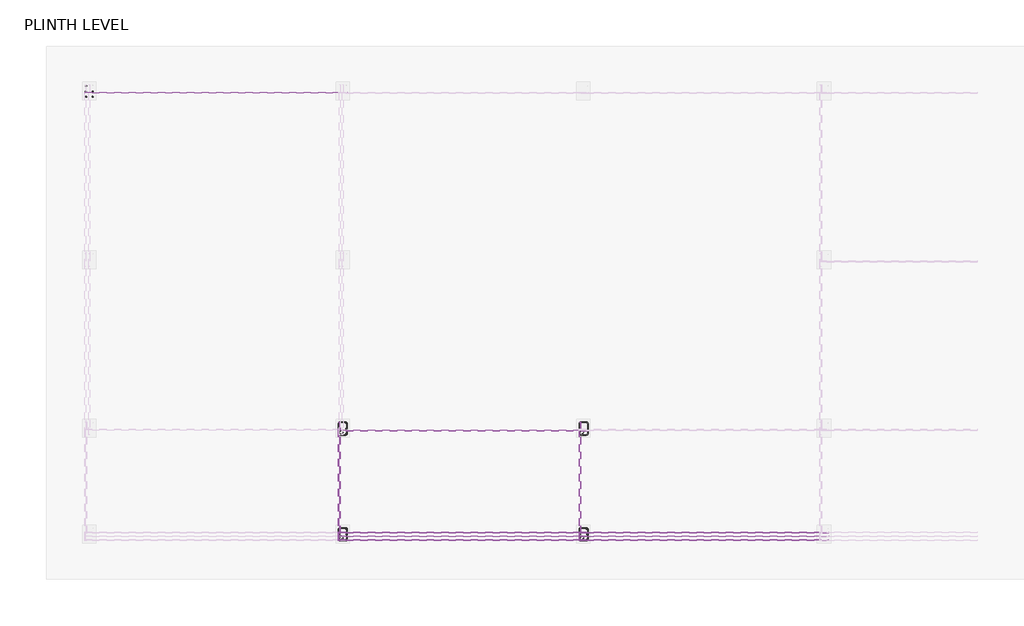
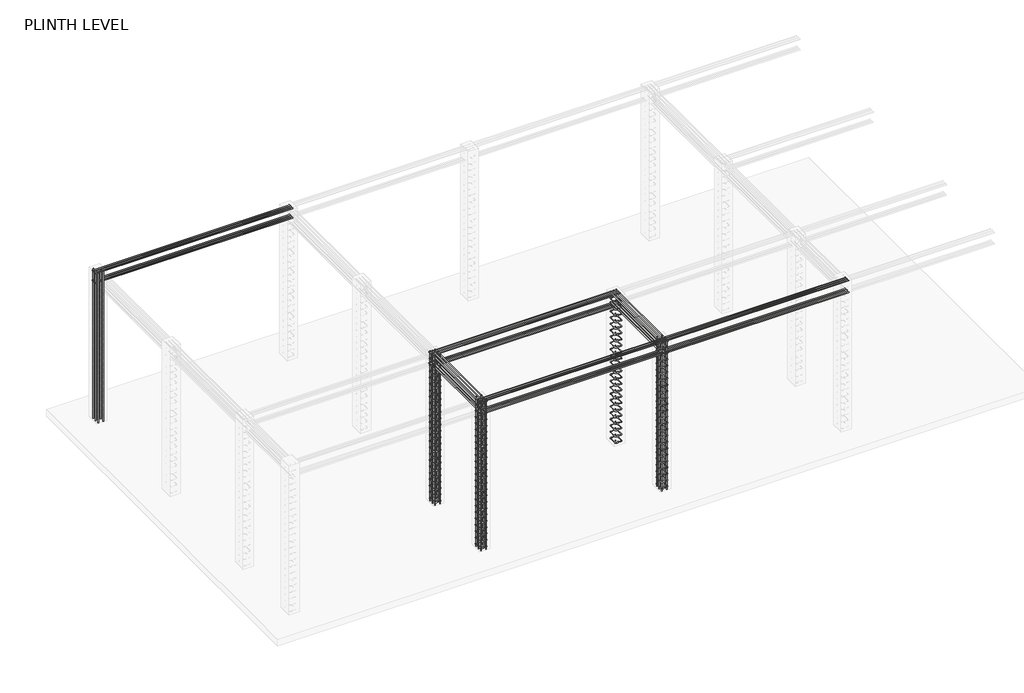
# One storey, part 3 of 6: 47 reinforcing bars.
"""IFC4 building model written with IfcOpenShell, lengths in millimetres."""

from ifc_helpers import new_model, si_unit, point, frame, origin, place, context, project, spatial, polyline, circle_curve, trimmed, segment, composite_curve, source, transform, mapped, element, save
from ifc_brep_helpers import swept_disk

model = new_model("IFC4")

# Units and contexts
model_context = context("Model", 3, world=origin())
ifc_project = project(units=[si_unit("LENGTHUNIT", "METRE", prefix="MILLI")], contexts=[model_context])

# Site, building, storey
site = spatial("IfcSite", under=ifc_project)
building = spatial("IfcBuilding", under=site)
storey = spatial("IfcBuildingStorey", under=building, Name="PLINTH LEVEL", Elevation=0.0)

# Reinforcing bars
placement = place(None, origin())
reinforcing_bar_shape = source(origin(), model_context, "Body", "SolidModel", [
    swept_disk(composite_curve([segment(polyline([(1580.248777, -15125.7150493, 44.0), (1546.3076515, -15159.6561748, 44.0)]), True, "CONTINUOUS"), segment(trimmed(circle_curve(frame((1563.2782143, -15176.6267376, 44.0), z_axis=(0.0, 0.0, 1.0), x_axis=(-16.970562799999925, 16.970562799999243, 0.0)), 24.0), [point((1546.3076515, -15159.6561748, 44.0))], [point((1563.2782143, -15200.6267376, 44.0))], True, "CARTESIAN"), True, "CONTINUOUS"), segment(polyline([(1563.2782143, -15200.6267376, 44.0), (1657.2782143, -15200.6267376, 44.0)]), True, "CONTINUOUS"), segment(trimmed(circle_curve(frame((1657.2782143, -15176.6267376, 44.0), z_axis=(0.0, 0.0, 1.0), x_axis=(0.0, -24.0, 0.0)), 24.0), [point((1657.2782143, -15200.6267376, 44.0))], [point((1681.2782143, -15176.6267376, 44.0))], True, "CARTESIAN"), True, "CONTINUOUS"), segment(polyline([(1681.2782143, -15176.6267376, 44.0), (1681.2782143, -15012.6267376, 44.0)]), True, "CONTINUOUS"), segment(trimmed(circle_curve(frame((1657.3162115, -15012.6267376, 42.650028), z_axis=(-0.05624883273897079, 0.0, 0.9984167811167355), x_axis=(23.962002799999937, 0.0, 1.349972000000001)), 24.0), [point((1681.2782143, -15012.6267376, 44.0))], [point((1657.3162115, -14988.6267376, 42.650028))], True, "CARTESIAN"), True, "CONTINUOUS"), segment(polyline([(1657.3162115, -14988.6267376, 42.650028), (1563.240217, -14988.6267376, 37.349972)]), True, "CONTINUOUS"), segment(trimmed(circle_curve(frame((1563.240217, -15012.6267376, 37.349972), z_axis=(-0.05624883273897079, 0.0, 0.9984167811167355), x_axis=(0.0, 24.0, 0.0)), 24.0), [point((1563.240217, -14988.6267376, 37.349972))], [point((1539.2782143, -15012.6267376, 36.0))], True, "CARTESIAN"), True, "CONTINUOUS"), segment(polyline([(1539.2782143, -15012.6267376, 36.0), (1539.2782143, -15176.6267376, 36.0)]), True, "CONTINUOUS"), segment(trimmed(circle_curve(frame((1563.2782143, -15176.6267376, 36.0), z_axis=(0.0, 0.0, 1.0), x_axis=(-24.0, 0.0, 0.0)), 24.0), [point((1539.2782143, -15176.6267376, 36.0))], [point((1580.248777, -15193.5973003, 36.0))], True, "CARTESIAN"), True, "CONTINUOUS"), segment(polyline([(1580.248777, -15193.5973003, 36.0), (1614.1899025, -15159.6561748, 36.0)]), True, "CONTINUOUS")], self_intersect=False), 4.0),
])
element("IfcReinforcingBar", 1, at=placement, inside=storey, context=model_context, shape_type="MappedRepresentation", body=[
    mapped(reinforcing_bar_shape, transform((0.0, 0.0, 0.0), x_axis=(1.0, 0.0, 0.0), y_axis=(0.0, 1.0, 0.0), z_axis=(0.0, 0.0, 1.0))),
    mapped(reinforcing_bar_shape, transform((0.0, 0.0, 149.0483786), x_axis=(1.0, 0.0, 0.0), y_axis=(0.0, 1.0, 0.0), z_axis=(0.0, 0.0, 1.0))),
    mapped(reinforcing_bar_shape, transform((0.0, 0.0, 298.0967572), x_axis=(1.0, 0.0, 0.0), y_axis=(0.0, 1.0, 0.0), z_axis=(0.0, 0.0, 1.0))),
    mapped(reinforcing_bar_shape, transform((0.0, 0.0, 447.1451358), x_axis=(1.0, 0.0, 0.0), y_axis=(0.0, 1.0, 0.0), z_axis=(0.0, 0.0, 1.0))),
    mapped(reinforcing_bar_shape, transform((0.0, 0.0, 596.1935144), x_axis=(1.0, 0.0, 0.0), y_axis=(0.0, 1.0, 0.0), z_axis=(0.0, 0.0, 1.0))),
    mapped(reinforcing_bar_shape, transform((0.0, 0.0, 745.241893), x_axis=(1.0, 0.0, 0.0), y_axis=(0.0, 1.0, 0.0), z_axis=(0.0, 0.0, 1.0))),
    mapped(reinforcing_bar_shape, transform((0.0, 0.0, 894.2902717), x_axis=(1.0, 0.0, 0.0), y_axis=(0.0, 1.0, 0.0), z_axis=(0.0, 0.0, 1.0))),
    mapped(reinforcing_bar_shape, transform((0.0, 0.0, 1043.3386503), x_axis=(1.0, 0.0, 0.0), y_axis=(0.0, 1.0, 0.0), z_axis=(0.0, 0.0, 1.0))),
    mapped(reinforcing_bar_shape, transform((0.0, 0.0, 1192.3870289), x_axis=(1.0, 0.0, 0.0), y_axis=(0.0, 1.0, 0.0), z_axis=(0.0, 0.0, 1.0))),
    mapped(reinforcing_bar_shape, transform((0.0, 0.0, 1341.4354075), x_axis=(1.0, 0.0, 0.0), y_axis=(0.0, 1.0, 0.0), z_axis=(0.0, 0.0, 1.0))),
    mapped(reinforcing_bar_shape, transform((0.0, 0.0, 1490.4837861), x_axis=(1.0, 0.0, 0.0), y_axis=(0.0, 1.0, 0.0), z_axis=(0.0, 0.0, 1.0))),
    mapped(reinforcing_bar_shape, transform((0.0, 0.0, 1639.5321647), x_axis=(1.0, 0.0, 0.0), y_axis=(0.0, 1.0, 0.0), z_axis=(0.0, 0.0, 1.0))),
    mapped(reinforcing_bar_shape, transform((0.0, 0.0, 1788.5805433), x_axis=(1.0, 0.0, 0.0), y_axis=(0.0, 1.0, 0.0), z_axis=(0.0, 0.0, 1.0))),
    mapped(reinforcing_bar_shape, transform((0.0, 0.0, 1937.6289219), x_axis=(1.0, 0.0, 0.0), y_axis=(0.0, 1.0, 0.0), z_axis=(0.0, 0.0, 1.0))),
    mapped(reinforcing_bar_shape, transform((0.0, 0.0, 2086.6773005), x_axis=(1.0, 0.0, 0.0), y_axis=(0.0, 1.0, 0.0), z_axis=(0.0, 0.0, 1.0))),
    mapped(reinforcing_bar_shape, transform((0.0, 0.0, 2235.7256791), x_axis=(1.0, 0.0, 0.0), y_axis=(0.0, 1.0, 0.0), z_axis=(0.0, 0.0, 1.0))),
    mapped(reinforcing_bar_shape, transform((0.0, 0.0, 2384.7740578), x_axis=(1.0, 0.0, 0.0), y_axis=(0.0, 1.0, 0.0), z_axis=(0.0, 0.0, 1.0))),
    mapped(reinforcing_bar_shape, transform((0.0, 0.0, 2533.8224364), x_axis=(1.0, 0.0, 0.0), y_axis=(0.0, 1.0, 0.0), z_axis=(0.0, 0.0, 1.0))),
    mapped(reinforcing_bar_shape, transform((0.0, 0.0, 2682.870815), x_axis=(1.0, 0.0, 0.0), y_axis=(0.0, 1.0, 0.0), z_axis=(0.0, 0.0, 1.0))),
    mapped(reinforcing_bar_shape, transform((0.0, 0.0, 2831.9191936), x_axis=(1.0, 0.0, 0.0), y_axis=(0.0, 1.0, 0.0), z_axis=(0.0, 0.0, 1.0))),
    mapped(reinforcing_bar_shape, transform((0.0, 0.0, 2980.9675722), x_axis=(1.0, 0.0, 0.0), y_axis=(0.0, 1.0, 0.0), z_axis=(0.0, 0.0, 1.0))),
    mapped(reinforcing_bar_shape, transform((0.0, 0.0, 3130.0159508), x_axis=(1.0, 0.0, 0.0), y_axis=(0.0, 1.0, 0.0), z_axis=(0.0, 0.0, 1.0))),
    mapped(reinforcing_bar_shape, transform((0.0, 0.0, 3279.0643294), x_axis=(1.0, 0.0, 0.0), y_axis=(0.0, 1.0, 0.0), z_axis=(0.0, 0.0, 1.0))),
])
element("IfcReinforcingBar", 2, at=placement, inside=storey, context=model_context, shape_type="SolidModel", body=[
    swept_disk(composite_curve([segment(polyline([(1665.7634957, -15004.1414562, -20.0), (1665.7634957, -15004.1414562, 3485.2)]), True, "CONTINUOUS")], self_intersect=False), 8.0),
])
element("IfcReinforcingBar", 3, at=placement, inside=storey, context=model_context, shape_type="SolidModel", body=[
    swept_disk(composite_curve([segment(polyline([(1665.7634957, -15185.112019, -20.0), (1665.7634957, -15185.112019, 3485.2)]), True, "CONTINUOUS")], self_intersect=False), 8.0),
])
element("IfcReinforcingBar", 4, at=placement, inside=storey, context=model_context, shape_type="SolidModel", body=[
    swept_disk(composite_curve([segment(polyline([(1669.2782143, -15094.6267376, -20.0), (1669.2782143, -15094.6267376, 3485.2)]), True, "CONTINUOUS")], self_intersect=False), 8.0),
])
element("IfcReinforcingBar", 5, at=placement, inside=storey, context=model_context, shape_type="SolidModel", body=[
    swept_disk(composite_curve([segment(polyline([(1554.7929329, -15004.1414562, -20.0), (1554.7929329, -15004.1414562, 3485.2)]), True, "CONTINUOUS")], self_intersect=False), 8.0),
])
element("IfcReinforcingBar", 6, at=placement, inside=storey, context=model_context, shape_type="SolidModel", body=[
    swept_disk(composite_curve([segment(polyline([(1554.7929329, -15185.112019, -20.0), (1554.7929329, -15185.112019, 3485.2)]), True, "CONTINUOUS")], self_intersect=False), 8.0),
])
element("IfcReinforcingBar", 7, at=placement, inside=storey, context=model_context, shape_type="SolidModel", body=[
    swept_disk(composite_curve([segment(polyline([(1551.2782143, -15094.6267376, -20.0), (1551.2782143, -15094.6267376, 3485.2)]), True, "CONTINUOUS")], self_intersect=False), 8.0),
])
reinforcing_bar_2_shape = source(origin(), model_context, "Body", "SolidModel", [
    swept_disk(composite_curve([segment(polyline([(5595.248777, -15125.7150493, 44.0), (5561.3076515, -15159.6561748, 44.0)]), True, "CONTINUOUS"), segment(trimmed(circle_curve(frame((5578.2782143, -15176.6267376, 44.0), z_axis=(0.0, 0.0, 1.0), x_axis=(-16.970562800000152, 16.970562799999243, 0.0)), 24.0), [point((5561.3076515, -15159.6561748, 44.0))], [point((5578.2782143, -15200.6267376, 44.0))], True, "CARTESIAN"), True, "CONTINUOUS"), segment(polyline([(5578.2782143, -15200.6267376, 44.0), (5672.2782143, -15200.6267376, 44.0)]), True, "CONTINUOUS"), segment(trimmed(circle_curve(frame((5672.2782143, -15176.6267376, 44.0), z_axis=(0.0, 0.0, 1.0), x_axis=(0.0, -24.0, 0.0)), 24.0), [point((5672.2782143, -15200.6267376, 44.0))], [point((5696.2782143, -15176.6267376, 44.0))], True, "CARTESIAN"), True, "CONTINUOUS"), segment(polyline([(5696.2782143, -15176.6267376, 44.0), (5696.2782143, -15012.6267376, 44.0)]), True, "CONTINUOUS"), segment(trimmed(circle_curve(frame((5672.3162115, -15012.6267376, 42.650028), z_axis=(-0.05624883273897079, 0.0, 0.9984167811167355), x_axis=(23.962002800000846, 0.0, 1.349972000000001)), 24.0), [point((5696.2782143, -15012.6267376, 44.0))], [point((5672.3162115, -14988.6267376, 42.650028))], True, "CARTESIAN"), True, "CONTINUOUS"), segment(polyline([(5672.3162115, -14988.6267376, 42.650028), (5578.240217, -14988.6267376, 37.349972)]), True, "CONTINUOUS"), segment(trimmed(circle_curve(frame((5578.240217, -15012.6267376, 37.349972), z_axis=(-0.05624883273897079, 0.0, 0.9984167811167355), x_axis=(0.0, 24.0, 0.0)), 24.0), [point((5578.240217, -14988.6267376, 37.349972))], [point((5554.2782143, -15012.6267376, 36.0))], True, "CARTESIAN"), True, "CONTINUOUS"), segment(polyline([(5554.2782143, -15012.6267376, 36.0), (5554.2782143, -15176.6267376, 36.0)]), True, "CONTINUOUS"), segment(trimmed(circle_curve(frame((5578.2782143, -15176.6267376, 36.0), z_axis=(0.0, 0.0, 1.0), x_axis=(-24.0, 0.0, 0.0)), 24.0), [point((5554.2782143, -15176.6267376, 36.0))], [point((5595.248777, -15193.5973003, 36.0))], True, "CARTESIAN"), True, "CONTINUOUS"), segment(polyline([(5595.248777, -15193.5973003, 36.0), (5629.1899025, -15159.6561748, 36.0)]), True, "CONTINUOUS")], self_intersect=False), 4.0),
])
element("IfcReinforcingBar", 8, at=placement, inside=storey, context=model_context, shape_type="MappedRepresentation", body=[
    mapped(reinforcing_bar_2_shape, transform((0.0, 0.0, 0.0), x_axis=(1.0, 0.0, 0.0), y_axis=(0.0, 1.0, 0.0), z_axis=(0.0, 0.0, 1.0))),
    mapped(reinforcing_bar_2_shape, transform((0.0, 0.0, 149.0483786), x_axis=(1.0, 0.0, 0.0), y_axis=(0.0, 1.0, 0.0), z_axis=(0.0, 0.0, 1.0))),
    mapped(reinforcing_bar_2_shape, transform((0.0, 0.0, 298.0967572), x_axis=(1.0, 0.0, 0.0), y_axis=(0.0, 1.0, 0.0), z_axis=(0.0, 0.0, 1.0))),
    mapped(reinforcing_bar_2_shape, transform((0.0, 0.0, 447.1451358), x_axis=(1.0, 0.0, 0.0), y_axis=(0.0, 1.0, 0.0), z_axis=(0.0, 0.0, 1.0))),
    mapped(reinforcing_bar_2_shape, transform((0.0, 0.0, 596.1935144), x_axis=(1.0, 0.0, 0.0), y_axis=(0.0, 1.0, 0.0), z_axis=(0.0, 0.0, 1.0))),
    mapped(reinforcing_bar_2_shape, transform((0.0, 0.0, 745.241893), x_axis=(1.0, 0.0, 0.0), y_axis=(0.0, 1.0, 0.0), z_axis=(0.0, 0.0, 1.0))),
    mapped(reinforcing_bar_2_shape, transform((0.0, 0.0, 894.2902717), x_axis=(1.0, 0.0, 0.0), y_axis=(0.0, 1.0, 0.0), z_axis=(0.0, 0.0, 1.0))),
    mapped(reinforcing_bar_2_shape, transform((0.0, 0.0, 1043.3386503), x_axis=(1.0, 0.0, 0.0), y_axis=(0.0, 1.0, 0.0), z_axis=(0.0, 0.0, 1.0))),
    mapped(reinforcing_bar_2_shape, transform((0.0, 0.0, 1192.3870289), x_axis=(1.0, 0.0, 0.0), y_axis=(0.0, 1.0, 0.0), z_axis=(0.0, 0.0, 1.0))),
    mapped(reinforcing_bar_2_shape, transform((0.0, 0.0, 1341.4354075), x_axis=(1.0, 0.0, 0.0), y_axis=(0.0, 1.0, 0.0), z_axis=(0.0, 0.0, 1.0))),
    mapped(reinforcing_bar_2_shape, transform((0.0, 0.0, 1490.4837861), x_axis=(1.0, 0.0, 0.0), y_axis=(0.0, 1.0, 0.0), z_axis=(0.0, 0.0, 1.0))),
    mapped(reinforcing_bar_2_shape, transform((0.0, 0.0, 1639.5321647), x_axis=(1.0, 0.0, 0.0), y_axis=(0.0, 1.0, 0.0), z_axis=(0.0, 0.0, 1.0))),
    mapped(reinforcing_bar_2_shape, transform((0.0, 0.0, 1788.5805433), x_axis=(1.0, 0.0, 0.0), y_axis=(0.0, 1.0, 0.0), z_axis=(0.0, 0.0, 1.0))),
    mapped(reinforcing_bar_2_shape, transform((0.0, 0.0, 1937.6289219), x_axis=(1.0, 0.0, 0.0), y_axis=(0.0, 1.0, 0.0), z_axis=(0.0, 0.0, 1.0))),
    mapped(reinforcing_bar_2_shape, transform((0.0, 0.0, 2086.6773005), x_axis=(1.0, 0.0, 0.0), y_axis=(0.0, 1.0, 0.0), z_axis=(0.0, 0.0, 1.0))),
    mapped(reinforcing_bar_2_shape, transform((0.0, 0.0, 2235.7256791), x_axis=(1.0, 0.0, 0.0), y_axis=(0.0, 1.0, 0.0), z_axis=(0.0, 0.0, 1.0))),
    mapped(reinforcing_bar_2_shape, transform((0.0, 0.0, 2384.7740578), x_axis=(1.0, 0.0, 0.0), y_axis=(0.0, 1.0, 0.0), z_axis=(0.0, 0.0, 1.0))),
    mapped(reinforcing_bar_2_shape, transform((0.0, 0.0, 2533.8224364), x_axis=(1.0, 0.0, 0.0), y_axis=(0.0, 1.0, 0.0), z_axis=(0.0, 0.0, 1.0))),
    mapped(reinforcing_bar_2_shape, transform((0.0, 0.0, 2682.870815), x_axis=(1.0, 0.0, 0.0), y_axis=(0.0, 1.0, 0.0), z_axis=(0.0, 0.0, 1.0))),
    mapped(reinforcing_bar_2_shape, transform((0.0, 0.0, 2831.9191936), x_axis=(1.0, 0.0, 0.0), y_axis=(0.0, 1.0, 0.0), z_axis=(0.0, 0.0, 1.0))),
    mapped(reinforcing_bar_2_shape, transform((0.0, 0.0, 2980.9675722), x_axis=(1.0, 0.0, 0.0), y_axis=(0.0, 1.0, 0.0), z_axis=(0.0, 0.0, 1.0))),
    mapped(reinforcing_bar_2_shape, transform((0.0, 0.0, 3130.0159508), x_axis=(1.0, 0.0, 0.0), y_axis=(0.0, 1.0, 0.0), z_axis=(0.0, 0.0, 1.0))),
    mapped(reinforcing_bar_2_shape, transform((0.0, 0.0, 3279.0643294), x_axis=(1.0, 0.0, 0.0), y_axis=(0.0, 1.0, 0.0), z_axis=(0.0, 0.0, 1.0))),
])
element("IfcReinforcingBar", 9, at=placement, inside=storey, context=model_context, shape_type="SolidModel", body=[
    swept_disk(composite_curve([segment(polyline([(5680.7634957, -15004.1414562, -20.0), (5680.7634957, -15004.1414562, 3485.2)]), True, "CONTINUOUS")], self_intersect=False), 8.0),
])
element("IfcReinforcingBar", 10, at=placement, inside=storey, context=model_context, shape_type="SolidModel", body=[
    swept_disk(composite_curve([segment(polyline([(5680.7634957, -15185.112019, -20.0), (5680.7634957, -15185.112019, 3485.2)]), True, "CONTINUOUS")], self_intersect=False), 8.0),
])
element("IfcReinforcingBar", 11, at=placement, inside=storey, context=model_context, shape_type="SolidModel", body=[
    swept_disk(composite_curve([segment(polyline([(5684.2782143, -15094.6267376, -20.0), (5684.2782143, -15094.6267376, 3485.2)]), True, "CONTINUOUS")], self_intersect=False), 8.0),
])
element("IfcReinforcingBar", 12, at=placement, inside=storey, context=model_context, shape_type="SolidModel", body=[
    swept_disk(composite_curve([segment(polyline([(5569.7929329, -15004.1414562, -20.0), (5569.7929329, -15004.1414562, 3485.2)]), True, "CONTINUOUS")], self_intersect=False), 8.0),
])
element("IfcReinforcingBar", 13, at=placement, inside=storey, context=model_context, shape_type="SolidModel", body=[
    swept_disk(composite_curve([segment(polyline([(5569.7929329, -15185.112019, -20.0), (5569.7929329, -15185.112019, 3485.2)]), True, "CONTINUOUS")], self_intersect=False), 8.0),
])
element("IfcReinforcingBar", 14, at=placement, inside=storey, context=model_context, shape_type="SolidModel", body=[
    swept_disk(composite_curve([segment(polyline([(5566.2782143, -15094.6267376, -20.0), (5566.2782143, -15094.6267376, 3485.2)]), True, "CONTINUOUS")], self_intersect=False), 8.0),
])
reinforcing_bar_3_shape = source(origin(), model_context, "Body", "SolidModel", [
    swept_disk(composite_curve([segment(polyline([(1580.248777, -13360.7150493, 44.0), (1546.3076515, -13394.6561748, 44.0)]), True, "CONTINUOUS"), segment(trimmed(circle_curve(frame((1563.2782143, -13411.6267376, 44.0), z_axis=(0.0, 0.0, 1.0), x_axis=(-16.970562799999925, 16.970562799999243, 0.0)), 24.0), [point((1546.3076515, -13394.6561748, 44.0))], [point((1563.2782143, -13435.6267376, 44.0))], True, "CARTESIAN"), True, "CONTINUOUS"), segment(polyline([(1563.2782143, -13435.6267376, 44.0), (1657.2782143, -13435.6267376, 44.0)]), True, "CONTINUOUS"), segment(trimmed(circle_curve(frame((1657.2782143, -13411.6267376, 44.0), z_axis=(0.0, 0.0, 1.0), x_axis=(0.0, -24.0, 0.0)), 24.0), [point((1657.2782143, -13435.6267376, 44.0))], [point((1681.2782143, -13411.6267376, 44.0))], True, "CARTESIAN"), True, "CONTINUOUS"), segment(polyline([(1681.2782143, -13411.6267376, 44.0), (1681.2782143, -13247.6267376, 44.0)]), True, "CONTINUOUS"), segment(trimmed(circle_curve(frame((1657.3162115, -13247.6267376, 42.650028), z_axis=(-0.05624883273897079, 0.0, 0.9984167811167355), x_axis=(23.962002799999937, 0.0, 1.349972000000001)), 24.0), [point((1681.2782143, -13247.6267376, 44.0))], [point((1657.3162115, -13223.6267376, 42.650028))], True, "CARTESIAN"), True, "CONTINUOUS"), segment(polyline([(1657.3162115, -13223.6267376, 42.650028), (1563.240217, -13223.6267376, 37.349972)]), True, "CONTINUOUS"), segment(trimmed(circle_curve(frame((1563.240217, -13247.6267376, 37.349972), z_axis=(-0.05624883273897079, 0.0, 0.9984167811167355), x_axis=(0.0, 24.0, 0.0)), 24.0), [point((1563.240217, -13223.6267376, 37.349972))], [point((1539.2782143, -13247.6267376, 36.0))], True, "CARTESIAN"), True, "CONTINUOUS"), segment(polyline([(1539.2782143, -13247.6267376, 36.0), (1539.2782143, -13411.6267376, 36.0)]), True, "CONTINUOUS"), segment(trimmed(circle_curve(frame((1563.2782143, -13411.6267376, 36.0), z_axis=(0.0, 0.0, 1.0), x_axis=(-24.0, 0.0, 0.0)), 24.0), [point((1539.2782143, -13411.6267376, 36.0))], [point((1580.248777, -13428.5973003, 36.0))], True, "CARTESIAN"), True, "CONTINUOUS"), segment(polyline([(1580.248777, -13428.5973003, 36.0), (1614.1899025, -13394.6561748, 36.0)]), True, "CONTINUOUS")], self_intersect=False), 4.0),
])
element("IfcReinforcingBar", 15, at=placement, inside=storey, context=model_context, shape_type="MappedRepresentation", body=[
    mapped(reinforcing_bar_3_shape, transform((0.0, 0.0, 0.0), x_axis=(1.0, 0.0, 0.0), y_axis=(0.0, 1.0, 0.0), z_axis=(0.0, 0.0, 1.0))),
    mapped(reinforcing_bar_3_shape, transform((0.0, 0.0, 149.0483786), x_axis=(1.0, 0.0, 0.0), y_axis=(0.0, 1.0, 0.0), z_axis=(0.0, 0.0, 1.0))),
    mapped(reinforcing_bar_3_shape, transform((0.0, 0.0, 298.0967572), x_axis=(1.0, 0.0, 0.0), y_axis=(0.0, 1.0, 0.0), z_axis=(0.0, 0.0, 1.0))),
    mapped(reinforcing_bar_3_shape, transform((0.0, 0.0, 447.1451358), x_axis=(1.0, 0.0, 0.0), y_axis=(0.0, 1.0, 0.0), z_axis=(0.0, 0.0, 1.0))),
    mapped(reinforcing_bar_3_shape, transform((0.0, 0.0, 596.1935144), x_axis=(1.0, 0.0, 0.0), y_axis=(0.0, 1.0, 0.0), z_axis=(0.0, 0.0, 1.0))),
    mapped(reinforcing_bar_3_shape, transform((0.0, 0.0, 745.241893), x_axis=(1.0, 0.0, 0.0), y_axis=(0.0, 1.0, 0.0), z_axis=(0.0, 0.0, 1.0))),
    mapped(reinforcing_bar_3_shape, transform((0.0, 0.0, 894.2902717), x_axis=(1.0, 0.0, 0.0), y_axis=(0.0, 1.0, 0.0), z_axis=(0.0, 0.0, 1.0))),
    mapped(reinforcing_bar_3_shape, transform((0.0, 0.0, 1043.3386503), x_axis=(1.0, 0.0, 0.0), y_axis=(0.0, 1.0, 0.0), z_axis=(0.0, 0.0, 1.0))),
    mapped(reinforcing_bar_3_shape, transform((0.0, 0.0, 1192.3870289), x_axis=(1.0, 0.0, 0.0), y_axis=(0.0, 1.0, 0.0), z_axis=(0.0, 0.0, 1.0))),
    mapped(reinforcing_bar_3_shape, transform((0.0, 0.0, 1341.4354075), x_axis=(1.0, 0.0, 0.0), y_axis=(0.0, 1.0, 0.0), z_axis=(0.0, 0.0, 1.0))),
    mapped(reinforcing_bar_3_shape, transform((0.0, 0.0, 1490.4837861), x_axis=(1.0, 0.0, 0.0), y_axis=(0.0, 1.0, 0.0), z_axis=(0.0, 0.0, 1.0))),
    mapped(reinforcing_bar_3_shape, transform((0.0, 0.0, 1639.5321647), x_axis=(1.0, 0.0, 0.0), y_axis=(0.0, 1.0, 0.0), z_axis=(0.0, 0.0, 1.0))),
    mapped(reinforcing_bar_3_shape, transform((0.0, 0.0, 1788.5805433), x_axis=(1.0, 0.0, 0.0), y_axis=(0.0, 1.0, 0.0), z_axis=(0.0, 0.0, 1.0))),
    mapped(reinforcing_bar_3_shape, transform((0.0, 0.0, 1937.6289219), x_axis=(1.0, 0.0, 0.0), y_axis=(0.0, 1.0, 0.0), z_axis=(0.0, 0.0, 1.0))),
    mapped(reinforcing_bar_3_shape, transform((0.0, 0.0, 2086.6773005), x_axis=(1.0, 0.0, 0.0), y_axis=(0.0, 1.0, 0.0), z_axis=(0.0, 0.0, 1.0))),
    mapped(reinforcing_bar_3_shape, transform((0.0, 0.0, 2235.7256791), x_axis=(1.0, 0.0, 0.0), y_axis=(0.0, 1.0, 0.0), z_axis=(0.0, 0.0, 1.0))),
    mapped(reinforcing_bar_3_shape, transform((0.0, 0.0, 2384.7740578), x_axis=(1.0, 0.0, 0.0), y_axis=(0.0, 1.0, 0.0), z_axis=(0.0, 0.0, 1.0))),
    mapped(reinforcing_bar_3_shape, transform((0.0, 0.0, 2533.8224364), x_axis=(1.0, 0.0, 0.0), y_axis=(0.0, 1.0, 0.0), z_axis=(0.0, 0.0, 1.0))),
    mapped(reinforcing_bar_3_shape, transform((0.0, 0.0, 2682.870815), x_axis=(1.0, 0.0, 0.0), y_axis=(0.0, 1.0, 0.0), z_axis=(0.0, 0.0, 1.0))),
    mapped(reinforcing_bar_3_shape, transform((0.0, 0.0, 2831.9191936), x_axis=(1.0, 0.0, 0.0), y_axis=(0.0, 1.0, 0.0), z_axis=(0.0, 0.0, 1.0))),
    mapped(reinforcing_bar_3_shape, transform((0.0, 0.0, 2980.9675722), x_axis=(1.0, 0.0, 0.0), y_axis=(0.0, 1.0, 0.0), z_axis=(0.0, 0.0, 1.0))),
    mapped(reinforcing_bar_3_shape, transform((0.0, 0.0, 3130.0159508), x_axis=(1.0, 0.0, 0.0), y_axis=(0.0, 1.0, 0.0), z_axis=(0.0, 0.0, 1.0))),
    mapped(reinforcing_bar_3_shape, transform((0.0, 0.0, 3279.0643294), x_axis=(1.0, 0.0, 0.0), y_axis=(0.0, 1.0, 0.0), z_axis=(0.0, 0.0, 1.0))),
])
element("IfcReinforcingBar", 16, at=placement, inside=storey, context=model_context, shape_type="SolidModel", body=[
    swept_disk(composite_curve([segment(polyline([(1665.7634957, -13239.1414562, -20.0), (1665.7634957, -13239.1414562, 3485.2)]), True, "CONTINUOUS")], self_intersect=False), 8.0),
])
element("IfcReinforcingBar", 17, at=placement, inside=storey, context=model_context, shape_type="SolidModel", body=[
    swept_disk(composite_curve([segment(polyline([(1665.7634957, -13420.112019, -20.0), (1665.7634957, -13420.112019, 3485.2)]), True, "CONTINUOUS")], self_intersect=False), 8.0),
])
element("IfcReinforcingBar", 18, at=placement, inside=storey, context=model_context, shape_type="SolidModel", body=[
    swept_disk(composite_curve([segment(polyline([(1669.2782143, -13329.6267376, -20.0), (1669.2782143, -13329.6267376, 3485.2)]), True, "CONTINUOUS")], self_intersect=False), 8.0),
])
element("IfcReinforcingBar", 19, at=placement, inside=storey, context=model_context, shape_type="SolidModel", body=[
    swept_disk(composite_curve([segment(polyline([(1554.7929329, -13239.1414562, -20.0), (1554.7929329, -13239.1414562, 3485.2)]), True, "CONTINUOUS")], self_intersect=False), 8.0),
])
element("IfcReinforcingBar", 20, at=placement, inside=storey, context=model_context, shape_type="SolidModel", body=[
    swept_disk(composite_curve([segment(polyline([(1554.7929329, -13420.112019, -20.0), (1554.7929329, -13420.112019, 3485.2)]), True, "CONTINUOUS")], self_intersect=False), 8.0),
])
element("IfcReinforcingBar", 21, at=placement, inside=storey, context=model_context, shape_type="SolidModel", body=[
    swept_disk(composite_curve([segment(polyline([(1551.2782143, -13329.6267376, -20.0), (1551.2782143, -13329.6267376, 3485.2)]), True, "CONTINUOUS")], self_intersect=False), 8.0),
])
reinforcing_bar_4_shape = source(origin(), model_context, "Body", "SolidModel", [
    swept_disk(composite_curve([segment(polyline([(5595.248777, -13360.7150493, 44.0), (5561.3076515, -13394.6561748, 44.0)]), True, "CONTINUOUS"), segment(trimmed(circle_curve(frame((5578.2782143, -13411.6267376, 44.0), z_axis=(0.0, 0.0, 1.0), x_axis=(-16.970562800000152, 16.970562799999243, 0.0)), 24.0), [point((5561.3076515, -13394.6561748, 44.0))], [point((5578.2782143, -13435.6267376, 44.0))], True, "CARTESIAN"), True, "CONTINUOUS"), segment(polyline([(5578.2782143, -13435.6267376, 44.0), (5672.2782143, -13435.6267376, 44.0)]), True, "CONTINUOUS"), segment(trimmed(circle_curve(frame((5672.2782143, -13411.6267376, 44.0), z_axis=(0.0, 0.0, 1.0), x_axis=(0.0, -24.0, 0.0)), 24.0), [point((5672.2782143, -13435.6267376, 44.0))], [point((5696.2782143, -13411.6267376, 44.0))], True, "CARTESIAN"), True, "CONTINUOUS"), segment(polyline([(5696.2782143, -13411.6267376, 44.0), (5696.2782143, -13247.6267376, 44.0)]), True, "CONTINUOUS"), segment(trimmed(circle_curve(frame((5672.3162115, -13247.6267376, 42.650028), z_axis=(-0.05624883273897079, 0.0, 0.9984167811167355), x_axis=(23.962002800000846, 0.0, 1.349972000000001)), 24.0), [point((5696.2782143, -13247.6267376, 44.0))], [point((5672.3162115, -13223.6267376, 42.650028))], True, "CARTESIAN"), True, "CONTINUOUS"), segment(polyline([(5672.3162115, -13223.6267376, 42.650028), (5578.240217, -13223.6267376, 37.349972)]), True, "CONTINUOUS"), segment(trimmed(circle_curve(frame((5578.240217, -13247.6267376, 37.349972), z_axis=(-0.05624883273897079, 0.0, 0.9984167811167355), x_axis=(0.0, 24.0, 0.0)), 24.0), [point((5578.240217, -13223.6267376, 37.349972))], [point((5554.2782143, -13247.6267376, 36.0))], True, "CARTESIAN"), True, "CONTINUOUS"), segment(polyline([(5554.2782143, -13247.6267376, 36.0), (5554.2782143, -13411.6267376, 36.0)]), True, "CONTINUOUS"), segment(trimmed(circle_curve(frame((5578.2782143, -13411.6267376, 36.0), z_axis=(0.0, 0.0, 1.0), x_axis=(-24.0, 0.0, 0.0)), 24.0), [point((5554.2782143, -13411.6267376, 36.0))], [point((5595.248777, -13428.5973003, 36.0))], True, "CARTESIAN"), True, "CONTINUOUS"), segment(polyline([(5595.248777, -13428.5973003, 36.0), (5629.1899025, -13394.6561748, 36.0)]), True, "CONTINUOUS")], self_intersect=False), 4.0),
])
element("IfcReinforcingBar", 22, at=placement, inside=storey, context=model_context, shape_type="MappedRepresentation", body=[
    mapped(reinforcing_bar_4_shape, transform((0.0, 0.0, 0.0), x_axis=(1.0, 0.0, 0.0), y_axis=(0.0, 1.0, 0.0), z_axis=(0.0, 0.0, 1.0))),
    mapped(reinforcing_bar_4_shape, transform((0.0, 0.0, 149.0483786), x_axis=(1.0, 0.0, 0.0), y_axis=(0.0, 1.0, 0.0), z_axis=(0.0, 0.0, 1.0))),
    mapped(reinforcing_bar_4_shape, transform((0.0, 0.0, 298.0967572), x_axis=(1.0, 0.0, 0.0), y_axis=(0.0, 1.0, 0.0), z_axis=(0.0, 0.0, 1.0))),
    mapped(reinforcing_bar_4_shape, transform((0.0, 0.0, 447.1451358), x_axis=(1.0, 0.0, 0.0), y_axis=(0.0, 1.0, 0.0), z_axis=(0.0, 0.0, 1.0))),
    mapped(reinforcing_bar_4_shape, transform((0.0, 0.0, 596.1935144), x_axis=(1.0, 0.0, 0.0), y_axis=(0.0, 1.0, 0.0), z_axis=(0.0, 0.0, 1.0))),
    mapped(reinforcing_bar_4_shape, transform((0.0, 0.0, 745.241893), x_axis=(1.0, 0.0, 0.0), y_axis=(0.0, 1.0, 0.0), z_axis=(0.0, 0.0, 1.0))),
    mapped(reinforcing_bar_4_shape, transform((0.0, 0.0, 894.2902717), x_axis=(1.0, 0.0, 0.0), y_axis=(0.0, 1.0, 0.0), z_axis=(0.0, 0.0, 1.0))),
    mapped(reinforcing_bar_4_shape, transform((0.0, 0.0, 1043.3386503), x_axis=(1.0, 0.0, 0.0), y_axis=(0.0, 1.0, 0.0), z_axis=(0.0, 0.0, 1.0))),
    mapped(reinforcing_bar_4_shape, transform((0.0, 0.0, 1192.3870289), x_axis=(1.0, 0.0, 0.0), y_axis=(0.0, 1.0, 0.0), z_axis=(0.0, 0.0, 1.0))),
    mapped(reinforcing_bar_4_shape, transform((0.0, 0.0, 1341.4354075), x_axis=(1.0, 0.0, 0.0), y_axis=(0.0, 1.0, 0.0), z_axis=(0.0, 0.0, 1.0))),
    mapped(reinforcing_bar_4_shape, transform((0.0, 0.0, 1490.4837861), x_axis=(1.0, 0.0, 0.0), y_axis=(0.0, 1.0, 0.0), z_axis=(0.0, 0.0, 1.0))),
    mapped(reinforcing_bar_4_shape, transform((0.0, 0.0, 1639.5321647), x_axis=(1.0, 0.0, 0.0), y_axis=(0.0, 1.0, 0.0), z_axis=(0.0, 0.0, 1.0))),
    mapped(reinforcing_bar_4_shape, transform((0.0, 0.0, 1788.5805433), x_axis=(1.0, 0.0, 0.0), y_axis=(0.0, 1.0, 0.0), z_axis=(0.0, 0.0, 1.0))),
    mapped(reinforcing_bar_4_shape, transform((0.0, 0.0, 1937.6289219), x_axis=(1.0, 0.0, 0.0), y_axis=(0.0, 1.0, 0.0), z_axis=(0.0, 0.0, 1.0))),
    mapped(reinforcing_bar_4_shape, transform((0.0, 0.0, 2086.6773005), x_axis=(1.0, 0.0, 0.0), y_axis=(0.0, 1.0, 0.0), z_axis=(0.0, 0.0, 1.0))),
    mapped(reinforcing_bar_4_shape, transform((0.0, 0.0, 2235.7256791), x_axis=(1.0, 0.0, 0.0), y_axis=(0.0, 1.0, 0.0), z_axis=(0.0, 0.0, 1.0))),
    mapped(reinforcing_bar_4_shape, transform((0.0, 0.0, 2384.7740578), x_axis=(1.0, 0.0, 0.0), y_axis=(0.0, 1.0, 0.0), z_axis=(0.0, 0.0, 1.0))),
    mapped(reinforcing_bar_4_shape, transform((0.0, 0.0, 2533.8224364), x_axis=(1.0, 0.0, 0.0), y_axis=(0.0, 1.0, 0.0), z_axis=(0.0, 0.0, 1.0))),
    mapped(reinforcing_bar_4_shape, transform((0.0, 0.0, 2682.870815), x_axis=(1.0, 0.0, 0.0), y_axis=(0.0, 1.0, 0.0), z_axis=(0.0, 0.0, 1.0))),
    mapped(reinforcing_bar_4_shape, transform((0.0, 0.0, 2831.9191936), x_axis=(1.0, 0.0, 0.0), y_axis=(0.0, 1.0, 0.0), z_axis=(0.0, 0.0, 1.0))),
    mapped(reinforcing_bar_4_shape, transform((0.0, 0.0, 2980.9675722), x_axis=(1.0, 0.0, 0.0), y_axis=(0.0, 1.0, 0.0), z_axis=(0.0, 0.0, 1.0))),
    mapped(reinforcing_bar_4_shape, transform((0.0, 0.0, 3130.0159508), x_axis=(1.0, 0.0, 0.0), y_axis=(0.0, 1.0, 0.0), z_axis=(0.0, 0.0, 1.0))),
    mapped(reinforcing_bar_4_shape, transform((0.0, 0.0, 3279.0643294), x_axis=(1.0, 0.0, 0.0), y_axis=(0.0, 1.0, 0.0), z_axis=(0.0, 0.0, 1.0))),
])
element("IfcReinforcingBar", 23, at=placement, inside=storey, context=model_context, shape_type="SolidModel", body=[
    swept_disk(composite_curve([segment(polyline([(-2564.2365043, -7790.112019, -20.0), (-2564.2365043, -7790.112019, 3485.2)]), True, "CONTINUOUS")], self_intersect=False), 8.0),
])
element("IfcReinforcingBar", 24, at=placement, inside=storey, context=model_context, shape_type="SolidModel", body=[
    swept_disk(composite_curve([segment(polyline([(-2560.7217857, -7699.6267376, -20.0), (-2560.7217857, -7699.6267376, 3485.2)]), True, "CONTINUOUS")], self_intersect=False), 8.0),
])
element("IfcReinforcingBar", 25, at=placement, inside=storey, context=model_context, shape_type="SolidModel", body=[
    swept_disk(composite_curve([segment(polyline([(-2675.2070671, -7609.1414562, -20.0), (-2675.2070671, -7609.1414562, 3485.2)]), True, "CONTINUOUS")], self_intersect=False), 8.0),
])
element("IfcReinforcingBar", 26, at=placement, inside=storey, context=model_context, shape_type="SolidModel", body=[
    swept_disk(composite_curve([segment(polyline([(-2675.2070671, -7790.112019, -20.0), (-2675.2070671, -7790.112019, 3485.2)]), True, "CONTINUOUS")], self_intersect=False), 8.0),
])
element("IfcReinforcingBar", 27, at=placement, inside=storey, context=model_context, shape_type="SolidModel", body=[
    swept_disk(composite_curve([segment(polyline([(-2678.7217857, -7699.6267376, -20.0), (-2678.7217857, -7699.6267376, 3485.2)]), True, "CONTINUOUS")], self_intersect=False), 8.0),
])
reinforcing_bar_5_shape = source(origin(), model_context, "Body", "SolidModel", [
    swept_disk(composite_curve([segment(polyline([(1677.2782143, -13219.6267376, 3463.45), (1677.2782143, -15204.6267376, 3463.45)]), True, "CONTINUOUS")], self_intersect=False), 8.0),
])
element("IfcReinforcingBar", 28, at=placement, inside=storey, context=model_context, shape_type="MappedRepresentation", body=[
    mapped(reinforcing_bar_5_shape, transform((0.0, 0.0, 0.0), x_axis=(1.0, 0.0, 0.0), y_axis=(0.0, 1.0, 0.0), z_axis=(0.0, 0.0, 1.0))),
    mapped(reinforcing_bar_5_shape, transform((-67.0, 0.0, 0.0), x_axis=(1.0, 0.0, 0.0), y_axis=(0.0, 1.0, 0.0), z_axis=(0.0, 0.0, 1.0))),
    mapped(reinforcing_bar_5_shape, transform((-134.0, 0.0, 0.0), x_axis=(1.0, 0.0, 0.0), y_axis=(0.0, 1.0, 0.0), z_axis=(0.0, 0.0, 1.0))),
])
reinforcing_bar_6_shape = source(origin(), model_context, "Body", "SolidModel", [
    swept_disk(composite_curve([segment(polyline([(1556.2071465, -13219.6267376, 3216.1289322), (1556.2071465, -15204.6267376, 3216.1289322)]), True, "CONTINUOUS")], self_intersect=False), 10.0),
])
element("IfcReinforcingBar", 29, at=placement, inside=storey, context=model_context, shape_type="MappedRepresentation", body=[
    mapped(reinforcing_bar_6_shape, transform((0.0, 0.0, 0.0), x_axis=(1.0, 0.0, 0.0), y_axis=(0.0, 1.0, 0.0), z_axis=(0.0, 0.0, 1.0))),
    mapped(reinforcing_bar_6_shape, transform((54.0710678, 0.0, 0.0), x_axis=(1.0, 0.0, 0.0), y_axis=(0.0, 1.0, 0.0), z_axis=(0.0, 0.0, 1.0))),
    mapped(reinforcing_bar_6_shape, transform((108.1421356, 0.0, 0.0), x_axis=(1.0, 0.0, 0.0), y_axis=(0.0, 1.0, 0.0), z_axis=(0.0, 0.0, 1.0))),
])
reinforcing_bar_7_shape = source(origin(), model_context, "Body", "SolidModel", [
    swept_disk(composite_curve([segment(polyline([(5692.2782143, -13219.6267376, 3463.45), (5692.2782143, -15204.6267376, 3463.45)]), True, "CONTINUOUS")], self_intersect=False), 8.0),
])
element("IfcReinforcingBar", 30, at=placement, inside=storey, context=model_context, shape_type="MappedRepresentation", body=[
    mapped(reinforcing_bar_7_shape, transform((0.0, 0.0, 0.0), x_axis=(1.0, 0.0, 0.0), y_axis=(0.0, 1.0, 0.0), z_axis=(0.0, 0.0, 1.0))),
    mapped(reinforcing_bar_7_shape, transform((-67.0, 0.0, 0.0), x_axis=(1.0, 0.0, 0.0), y_axis=(0.0, 1.0, 0.0), z_axis=(0.0, 0.0, 1.0))),
    mapped(reinforcing_bar_7_shape, transform((-134.0, 0.0, 0.0), x_axis=(1.0, 0.0, 0.0), y_axis=(0.0, 1.0, 0.0), z_axis=(0.0, 0.0, 1.0))),
])
reinforcing_bar_8_shape = source(origin(), model_context, "Body", "SolidModel", [
    swept_disk(composite_curve([segment(polyline([(5571.2071465, -13219.6267376, 3216.1289322), (5571.2071465, -15204.6267376, 3216.1289322)]), True, "CONTINUOUS")], self_intersect=False), 10.0),
])
element("IfcReinforcingBar", 31, at=placement, inside=storey, context=model_context, shape_type="MappedRepresentation", body=[
    mapped(reinforcing_bar_8_shape, transform((0.0, 0.0, 0.0), x_axis=(1.0, 0.0, 0.0), y_axis=(0.0, 1.0, 0.0), z_axis=(0.0, 0.0, 1.0))),
    mapped(reinforcing_bar_8_shape, transform((54.0710678, 0.0, 0.0), x_axis=(1.0, 0.0, 0.0), y_axis=(0.0, 1.0, 0.0), z_axis=(0.0, 0.0, 1.0))),
    mapped(reinforcing_bar_8_shape, transform((108.1421356, 0.0, 0.0), x_axis=(1.0, 0.0, 0.0), y_axis=(0.0, 1.0, 0.0), z_axis=(0.0, 0.0, 1.0))),
])
reinforcing_bar_9_shape = source(origin(), model_context, "Body", "SolidModel", [
    swept_disk(composite_curve([segment(polyline([(5700.2782143, -13361.9489767, 3462.825), (1535.2782143, -13361.9489767, 3462.825)]), True, "CONTINUOUS")], self_intersect=False), 8.0),
])
element("IfcReinforcingBar", 32, at=placement, inside=storey, context=model_context, shape_type="MappedRepresentation", body=[
    mapped(reinforcing_bar_9_shape, transform((0.0, 0.0, 0.0), x_axis=(1.0, 0.0, 0.0), y_axis=(0.0, 1.0, 0.0), z_axis=(0.0, 0.0, 1.0))),
    mapped(reinforcing_bar_9_shape, transform((0.0, 67.1611195, 0.0), x_axis=(1.0, 0.0, 0.0), y_axis=(0.0, 1.0, 0.0), z_axis=(0.0, 0.0, 1.0))),
    mapped(reinforcing_bar_9_shape, transform((0.0, 134.3222391, 0.0), x_axis=(1.0, 0.0, 0.0), y_axis=(0.0, 1.0, 0.0), z_axis=(0.0, 0.0, 1.0))),
])
reinforcing_bar_10_shape = source(origin(), model_context, "Body", "SolidModel", [
    swept_disk(composite_curve([segment(polyline([(5700.2782143, -13229.6267376, 3201.1289322), (1535.2782143, -13229.6267376, 3201.1289322)]), True, "CONTINUOUS")], self_intersect=False), 10.0),
])
element("IfcReinforcingBar", 33, at=placement, inside=storey, context=model_context, shape_type="MappedRepresentation", body=[
    mapped(reinforcing_bar_10_shape, transform((0.0, 0.0, 0.0), x_axis=(1.0, 0.0, 0.0), y_axis=(0.0, 1.0, 0.0), z_axis=(0.0, 0.0, 1.0))),
    mapped(reinforcing_bar_10_shape, transform((0.0, -67.0355339, 0.0), x_axis=(1.0, 0.0, 0.0), y_axis=(0.0, 1.0, 0.0), z_axis=(0.0, 0.0, 1.0))),
    mapped(reinforcing_bar_10_shape, transform((0.0, -134.0710678, 0.0), x_axis=(1.0, 0.0, 0.0), y_axis=(0.0, 1.0, 0.0), z_axis=(0.0, 0.0, 1.0))),
])
reinforcing_bar_11_shape = source(origin(), model_context, "Body", "SolidModel", [
    swept_disk(composite_curve([segment(polyline([(1685.2782143, -7720.112019, 3445.6852814), (-2694.7217857, -7720.112019, 3445.6852814)]), True, "CONTINUOUS")], self_intersect=False), 8.0),
])
element("IfcReinforcingBar", 34, at=placement, inside=storey, context=model_context, shape_type="MappedRepresentation", body=[
    mapped(reinforcing_bar_11_shape, transform((0.0, 0.0, 0.0), x_axis=(1.0, 0.0, 0.0), y_axis=(0.0, 1.0, 0.0), z_axis=(0.0, 0.0, 1.0))),
    mapped(reinforcing_bar_11_shape, transform((0.0, 55.4852814, 0.0), x_axis=(1.0, 0.0, 0.0), y_axis=(0.0, 1.0, 0.0), z_axis=(0.0, 0.0, 1.0))),
    mapped(reinforcing_bar_11_shape, transform((0.0, 110.9705627, 0.0), x_axis=(1.0, 0.0, 0.0), y_axis=(0.0, 1.0, 0.0), z_axis=(0.0, 0.0, 1.0))),
])
reinforcing_bar_12_shape = source(origin(), model_context, "Body", "SolidModel", [
    swept_disk(composite_curve([segment(polyline([(1685.2782143, -7607.6267376, 3223.2), (-2694.7217857, -7607.6267376, 3223.2)]), True, "CONTINUOUS")], self_intersect=False), 10.0),
])
element("IfcReinforcingBar", 35, at=placement, inside=storey, context=model_context, shape_type="MappedRepresentation", body=[
    mapped(reinforcing_bar_12_shape, transform((0.0, 0.0, 0.0), x_axis=(1.0, 0.0, 0.0), y_axis=(0.0, 1.0, 0.0), z_axis=(0.0, 0.0, 1.0))),
    mapped(reinforcing_bar_12_shape, transform((0.0, -55.5355339, 0.0), x_axis=(1.0, 0.0, 0.0), y_axis=(0.0, 1.0, 0.0), z_axis=(0.0, 0.0, 1.0))),
    mapped(reinforcing_bar_12_shape, transform((0.0, -111.0710678, 0.0), x_axis=(1.0, 0.0, 0.0), y_axis=(0.0, 1.0, 0.0), z_axis=(0.0, 0.0, 1.0))),
])
element("IfcReinforcingBar", 36, at=placement, inside=storey, context=model_context, shape_type="SolidModel", body=[
    swept_disk(composite_curve([segment(polyline([(9715.2782143, -15185.1473743, 3465.7206367), (5550.2782143, -15185.1473743, 3465.7206367)]), True, "CONTINUOUS")], self_intersect=False), 7.95),
])
element("IfcReinforcingBar", 37, at=placement, inside=storey, context=model_context, shape_type="SolidModel", body=[
    swept_disk(composite_curve([segment(polyline([(9715.2782143, -15064.8346024, 3198.6289322), (5550.2782143, -15064.8346024, 3198.6289322)]), True, "CONTINUOUS")], self_intersect=False), 10.0),
])
element("IfcReinforcingBar", 38, at=placement, inside=storey, context=model_context, shape_type="SolidModel", body=[
    swept_disk(composite_curve([segment(polyline([(9715.2782143, -15129.6267376, 3465.2), (5550.2782143, -15129.6267376, 3465.2)]), True, "CONTINUOUS")], self_intersect=False), 7.95),
])
element("IfcReinforcingBar", 39, at=placement, inside=storey, context=model_context, shape_type="SolidModel", body=[
    swept_disk(composite_curve([segment(polyline([(9715.2782143, -15074.1061009, 3465.7206367), (5550.2782143, -15074.1061009, 3465.7206367)]), True, "CONTINUOUS")], self_intersect=False), 7.95),
])
element("IfcReinforcingBar", 40, at=placement, inside=storey, context=model_context, shape_type="SolidModel", body=[
    swept_disk(composite_curve([segment(polyline([(9715.2782143, -15129.6267376, 3198.6289322), (5550.2782143, -15129.6267376, 3198.6289322)]), True, "CONTINUOUS")], self_intersect=False), 10.0),
])
element("IfcReinforcingBar", 41, at=placement, inside=storey, context=model_context, shape_type="SolidModel", body=[
    swept_disk(composite_curve([segment(polyline([(9715.2782143, -15194.6267376, 3198.6289322), (5550.2782143, -15194.6267376, 3198.6289322)]), True, "CONTINUOUS")], self_intersect=False), 10.0),
])
element("IfcReinforcingBar", 42, at=placement, inside=storey, context=model_context, shape_type="SolidModel", body=[
    swept_disk(composite_curve([segment(polyline([(5700.2782143, -15185.1473743, 3465.7206367), (1535.2782143, -15185.1473743, 3465.7206367)]), True, "CONTINUOUS")], self_intersect=False), 7.95),
])
element("IfcReinforcingBar", 43, at=placement, inside=storey, context=model_context, shape_type="SolidModel", body=[
    swept_disk(composite_curve([segment(polyline([(5700.2782143, -15064.8346024, 3198.6289322), (1535.2782143, -15064.8346024, 3198.6289322)]), True, "CONTINUOUS")], self_intersect=False), 10.0),
])
element("IfcReinforcingBar", 44, at=placement, inside=storey, context=model_context, shape_type="SolidModel", body=[
    swept_disk(composite_curve([segment(polyline([(5700.2782143, -15129.6267376, 3465.2), (1535.2782143, -15129.6267376, 3465.2)]), True, "CONTINUOUS")], self_intersect=False), 7.95),
])
element("IfcReinforcingBar", 45, at=placement, inside=storey, context=model_context, shape_type="SolidModel", body=[
    swept_disk(composite_curve([segment(polyline([(5700.2782143, -15074.1061009, 3465.7206367), (1535.2782143, -15074.1061009, 3465.7206367)]), True, "CONTINUOUS")], self_intersect=False), 7.95),
])
element("IfcReinforcingBar", 46, at=placement, inside=storey, context=model_context, shape_type="SolidModel", body=[
    swept_disk(composite_curve([segment(polyline([(5700.2782143, -15129.6267376, 3198.6289322), (1535.2782143, -15129.6267376, 3198.6289322)]), True, "CONTINUOUS")], self_intersect=False), 10.0),
])
element("IfcReinforcingBar", 47, at=placement, inside=storey, context=model_context, shape_type="SolidModel", body=[
    swept_disk(composite_curve([segment(polyline([(5700.2782143, -15194.6267376, 3198.6289322), (1535.2782143, -15194.6267376, 3198.6289322)]), True, "CONTINUOUS")], self_intersect=False), 10.0),
])

save(model, "model.ifc")

# Revit data of these elements
# Elements 1, 2, 3, 4, 5, 6, 7, 8, 9, 10, 11, 12, 13, 14, 15, 16, 17, 18, 19, 20, 21, 22, 23, 24, 25, 26, 27, 28, 29, 30, 31, 32, 33, 34, 35, 36, 37, 38, 39, 40, 41, 42, 43, 44, 45, 46, 47 (IfcReinforcingBar)
#   Phase Created = New Construction
